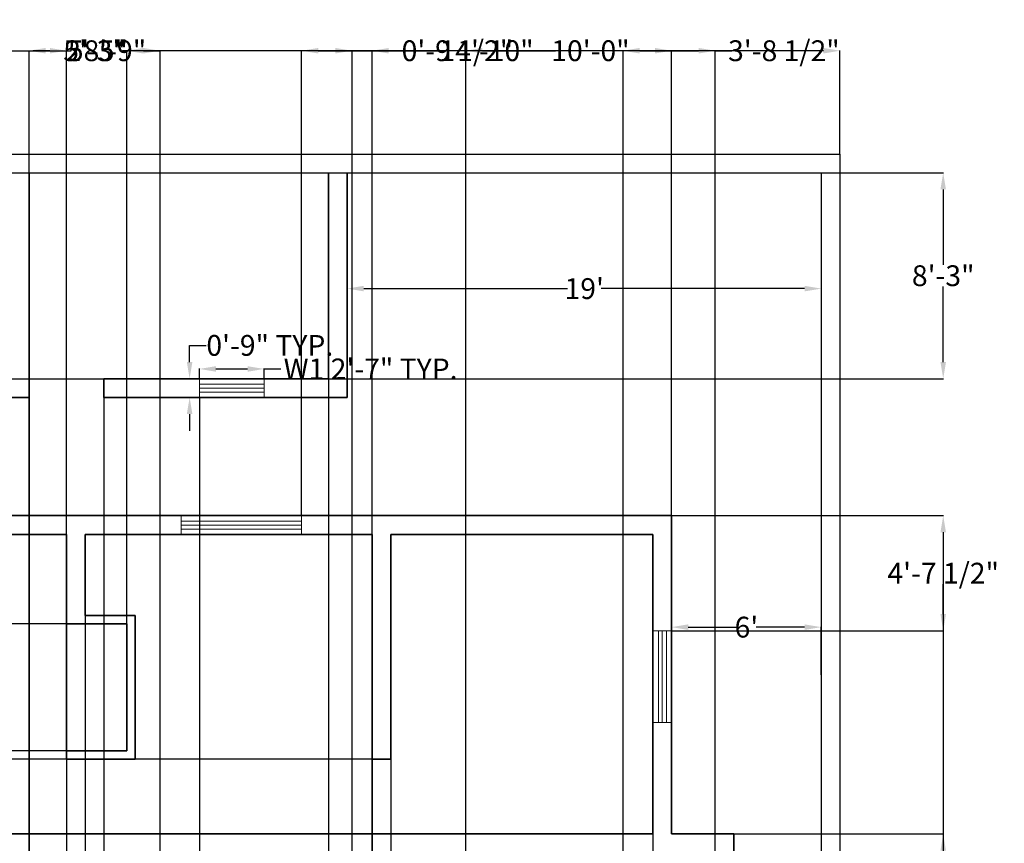
# Model space of a CAD drawing. Units: inches. Extents: x -63 to 800, y 3068 to 4133.
# Tile 5 of 5: x 327 to 800, y 3737 to 4133. Entities that reach past the tile are written whole.
import ezdxf

# ---------------------------------------------------------------- set-up
doc = ezdxf.new("R2010")
doc.units = ezdxf.units.IN
doc.header["$MEASUREMENT"] = 0
for name, color, linetype, lineweight in [('A-ANNO-DIMS', 2, 'Continuous', 13), ('A-GLAZ', 4, 'Continuous', 18), ('A-WALL', 7, 'Continuous', 35), ('A-WALL-SITE', 8, 'Continuous', 30)]:
    doc.layers.add(name, color=color, linetype=linetype, lineweight=lineweight)
doc.styles.get("Standard").update_dxf_attribs({"font": 'arial.ttf'})
doc.dimstyles.get("Standard").update_dxf_attribs({"dimtxt": 10, "dimasz": 8, "dimexe": 0.18, "dimexo": 0.0625, "dimgap": 0.09, "dimtad": 0, "dimtih": 1, "dimtoh": 1, "dimdec": 0, "dimzin": 0, "dimdsep": 46, "dimlunit": 3, "dimtxsty": 'Standard', "dimcen": 0.09, "dimadec": 0, "dimazin": 0, "dimtfac": 1, "dimtdec": 0, "dimtofl": 0, "dimtmove": 0, "dimatfit": 3, "dimfxl": 1, "dimtolj": 1, "dimtzin": 0, "dimarcsym": 0})

# ---------------------------------------------------------------- blocks, each defined once
blk = doc.blocks.new('*D1')
at = {"layer": 'A-ANNO-DIMS', "color": 0, "lineweight": -2, "transparency": 16777216}
for p, q in [((484.31, 4004.22), (484.31, 4003.78)), ((492.31, 4003.96), (590.2, 4003.96)), ((704.31, 4003.96), (606.41, 4003.96)), ((712.31, 4004.22), (712.31, 4003.78))]:
    blk.add_line(p, q, dxfattribs=at)
at = {"layer": 'A-ANNO-DIMS', "color": 0, "transparency": 16777216}
for points in [[(492.31, 4005.3), (492.31, 4002.63), (484.31, 4003.96)], [(704.31, 4005.3), (704.31, 4002.63), (712.31, 4003.96)]]:
    blk.add_solid(points, dxfattribs=at)
at = {"layer": 'Defpoints', "color": 0, "transparency": 16777216}
for p in [(484.31, 4004.28), (712.31, 4004.28), (712.31, 4003.96)]:
    blk.add_point(p, dxfattribs=at)
at = {"layer": 'A-ANNO-DIMS', "color": 0, "transparency": 16777216, "insert": (598.31, 4003.96), "char_height": 10, "attachment_point": 5}
blk.add_mtext("\\A1;19'", dxfattribs=at)
blk = doc.blocks.new('*D4')
at = {"layer": 'A-ANNO-DIMS', "color": 0, "lineweight": -2, "transparency": 16777216}
for p, q in [((640.31, 3818.37), (640.31, 3841.4)), ((648.31, 3841.22), (671.59, 3841.22)), ((704.31, 3841.22), (681.03, 3841.22)), ((712.31, 3818.37), (712.31, 3841.4))]:
    blk.add_line(p, q, dxfattribs=at)
at = {"layer": 'A-ANNO-DIMS', "color": 0, "transparency": 16777216}
for points in [[(648.31, 3842.55), (648.31, 3839.89), (640.31, 3841.22)], [(704.31, 3842.55), (704.31, 3839.89), (712.31, 3841.22)]]:
    blk.add_solid(points, dxfattribs=at)
at = {"layer": 'Defpoints', "color": 0, "transparency": 16777216}
for p in [(712.31, 3841.22), (640.31, 3818.31), (712.31, 3818.31)]:
    blk.add_point(p, dxfattribs=at)
at = {"layer": 'A-ANNO-DIMS', "color": 0, "transparency": 16777216, "insert": (676.31, 3841.22), "char_height": 10, "attachment_point": 5}
blk.add_mtext("\\A1;6'", dxfattribs=at)
blk = doc.blocks.new('WIN-31')
blk.add_lwpolyline([(0, 9), (31.17, 9), (31.17, 0), (0, 0)], close=True)
blk.add_lwpolyline([(0, 4.5), (31.17, 4.5), (31.17, 6.29), (0, 6.29), (0, 2.51), (31.17, 2.51)])
blk = doc.blocks.new('WIN-44')
blk.add_lwpolyline([(0, 0), (0, 44.17), (9, 44.17), (9, 0)], close=True)
for points in [[(2.71, 44.17), (2.71, 0), (6.5, 0), (6.5, 44.17)], [(4.5, 0), (4.5, 44.17)]]:
    blk.add_lwpolyline(points)
blk = doc.blocks.new('WIN-58')
blk.add_lwpolyline([(0, 9), (57.99, 9), (57.99, 0), (0, 0)], close=True)
for points in [[(0, 4.5), (57.99, 4.5), (57.99, 6.29), (0, 6.29)], [(0, 2.51), (57.99, 2.51)]]:
    blk.add_lwpolyline(points)
blk = doc.blocks.new('*D13')
at = {"layer": 'A-ANNO-DIMS', "color": 0, "lineweight": -2, "transparency": 16777216}
for p, q in [((413.21, 3960.72), (413.21, 3965.52)), ((421.21, 3965.34), (436.38, 3965.34)), ((444.38, 3960.72), (444.38, 3965.52)), ((444.38, 3965.34), (452.38, 3965.34))]:
    blk.add_line(p, q, dxfattribs=at)
at = {"layer": 'A-ANNO-DIMS', "color": 0, "transparency": 16777216}
for points in [[(421.21, 3966.67), (421.21, 3964), (413.21, 3965.34)], [(436.38, 3966.67), (436.38, 3964), (444.38, 3965.34)]]:
    blk.add_solid(points, dxfattribs=at)
at = {"layer": 'Defpoints', "color": 0, "transparency": 16777216}
for p in [(444.38, 3965.34), (413.21, 3960.66), (444.38, 3960.66)]:
    blk.add_point(p, dxfattribs=at)
at = {"layer": 'A-ANNO-DIMS', "color": 0, "transparency": 16777216, "insert": (495.58, 3965.34), "char_height": 10, "attachment_point": 5}
blk.add_mtext('\\A1;W1 2\'-7" TYP.', dxfattribs=at)
blk = doc.blocks.new('*D14')
at = {"layer": 'A-ANNO-DIMS', "color": 0, "lineweight": -2, "transparency": 16777216}
for p, q in [((408.54, 3968.66), (408.54, 3976.66)), ((408.54, 3976.66), (416.54, 3976.66)), ((413.15, 3960.66), (408.36, 3960.66)), ((413.15, 3951.66), (408.36, 3951.66)), ((408.54, 3943.66), (408.54, 3935.66))]:
    blk.add_line(p, q, dxfattribs=at)
at = {"layer": 'A-ANNO-DIMS', "color": 0, "transparency": 16777216}
for points in [[(407.2, 3968.66), (409.87, 3968.66), (408.54, 3960.66)], [(407.2, 3943.66), (409.87, 3943.66), (408.54, 3951.66)]]:
    blk.add_solid(points, dxfattribs=at)
at = {"layer": 'Defpoints', "color": 0, "transparency": 16777216}
for p in [(408.54, 3960.66), (413.21, 3960.66), (413.21, 3951.66)]:
    blk.add_point(p, dxfattribs=at)
at = {"layer": 'A-ANNO-DIMS', "color": 0, "transparency": 16777216, "insert": (447.1, 3976.66), "char_height": 10, "attachment_point": 5}
blk.add_mtext('\\A1;0\'-9" TYP.', dxfattribs=at)
blk = doc.blocks.new('*D19')
at = {"layer": 'A-ANNO-DIMS', "color": 0, "lineweight": -2, "transparency": 16777216}
for p, q in [((16.31, 4068.72), (16.31, 4118.49)), ((24.31, 4118.31), (351.54, 4118.31)), ((713.31, 4118.31), (386.08, 4118.31)), ((721.31, 4068.72), (721.31, 4118.49))]:
    blk.add_line(p, q, dxfattribs=at)
at = {"layer": 'A-ANNO-DIMS', "color": 0, "transparency": 16777216}
for points in [[(24.31, 4119.64), (24.31, 4116.98), (16.31, 4118.31)], [(713.31, 4119.64), (713.31, 4116.98), (721.31, 4118.31)]]:
    blk.add_solid(points, dxfattribs=at)
at = {"layer": 'Defpoints', "color": 0, "transparency": 16777216}
for p in [(721.31, 4118.31), (16.31, 4068.66), (721.31, 4068.66)]:
    blk.add_point(p, dxfattribs=at)
at = {"layer": 'A-ANNO-DIMS', "color": 0, "transparency": 16777216, "insert": (368.81, 4118.31), "char_height": 10, "attachment_point": 5}
blk.add_mtext('\\A1;58\'-9"', dxfattribs=at)
blk = doc.blocks.new('*D25')
at = {"layer": 'A-ANNO-DIMS', "color": 0, "lineweight": -2, "transparency": 16777216}
for p, q in [((331.31, 4059.6), (331.31, 3082.48)), ((475.31, 4059.6), (475.31, 3082.48)), ((339.31, 3082.66), (386.51, 3082.66)), ((467.31, 3082.66), (420.1, 3082.66))]:
    blk.add_line(p, q, dxfattribs=at)
at = {"layer": 'A-ANNO-DIMS', "color": 0, "transparency": 16777216}
for points in [[(339.31, 3083.99), (339.31, 3081.33), (331.31, 3082.66)], [(467.31, 3083.99), (467.31, 3081.33), (475.31, 3082.66)]]:
    blk.add_solid(points, dxfattribs=at)
at = {"layer": 'Defpoints', "color": 0, "transparency": 16777216}
for p in [(331.31, 4059.66), (475.31, 4059.66), (475.31, 3082.66)]:
    blk.add_point(p, dxfattribs=at)
at = {"layer": 'A-ANNO-DIMS', "color": 0, "transparency": 16777216, "insert": (403.31, 3082.66), "char_height": 10, "attachment_point": 5}
blk.add_mtext('\\A1;12\'-0"', dxfattribs=at)
blk = doc.blocks.new('*D26')
at = {"layer": 'A-ANNO-DIMS', "color": 0, "lineweight": -2, "transparency": 16777216}
for p, q in [((25.37, 4059.66), (771.14, 4059.66)), ((770.96, 4051.66), (770.96, 4015.36)), ((770.96, 3968.66), (770.96, 4004.96)), ((25.37, 3960.66), (771.14, 3960.66))]:
    blk.add_line(p, q, dxfattribs=at)
at = {"layer": 'A-ANNO-DIMS', "color": 0, "transparency": 16777216}
for points in [[(769.63, 4051.66), (772.29, 4051.66), (770.96, 4059.66)], [(769.63, 3968.66), (772.29, 3968.66), (770.96, 3960.66)]]:
    blk.add_solid(points, dxfattribs=at)
at = {"layer": 'Defpoints', "color": 0, "transparency": 16777216}
for p in [(25.31, 4059.66), (770.96, 4059.66), (25.31, 3960.66)]:
    blk.add_point(p, dxfattribs=at)
at = {"layer": 'A-ANNO-DIMS', "color": 0, "transparency": 16777216, "insert": (770.96, 4010.16), "char_height": 10, "attachment_point": 5}
blk.add_mtext('\\A1;8\'-3"', dxfattribs=at)
blk = doc.blocks.new('*D28')
at = {"layer": 'A-ANNO-DIMS', "color": 0, "lineweight": -2, "transparency": 16777216}
for p, q in [((297.16, 3951.55), (297.16, 3082.48)), ((331.31, 3951.6), (331.31, 3082.48)), ((305.16, 3082.66), (323.31, 3082.66)), ((331.31, 3082.66), (339.31, 3082.66))]:
    blk.add_line(p, q, dxfattribs=at)
at = {"layer": 'A-ANNO-DIMS', "color": 0, "transparency": 16777216}
for points in [[(305.16, 3083.99), (305.16, 3081.33), (297.16, 3082.66)], [(323.31, 3083.99), (323.31, 3081.33), (331.31, 3082.66)]]:
    blk.add_solid(points, dxfattribs=at)
at = {"layer": 'Defpoints', "color": 0, "transparency": 16777216}
for p in [(297.16, 3951.61), (331.31, 3951.66), (331.31, 3082.66)]:
    blk.add_point(p, dxfattribs=at)
at = {"layer": 'A-ANNO-DIMS', "color": 0, "transparency": 16777216, "insert": (356.66, 3082.66), "char_height": 10, "attachment_point": 5}
blk.add_mtext('\\A1;2\'-10"', dxfattribs=at)
blk = doc.blocks.new('*D29')
at = {"layer": 'A-ANNO-DIMS', "color": 0, "lineweight": -2, "transparency": 16777216}
for p, q in [((367.31, 3951.6), (367.31, 3082.48)), ((413.21, 3951.6), (413.21, 3082.48)), ((359.31, 3082.66), (351.31, 3082.66)), ((421.21, 3082.66), (429.21, 3082.66))]:
    blk.add_line(p, q, dxfattribs=at)
at = {"layer": 'A-ANNO-DIMS', "color": 0, "transparency": 16777216}
for points in [[(359.31, 3083.99), (359.31, 3081.33), (367.31, 3082.66)], [(421.21, 3083.99), (421.21, 3081.33), (413.21, 3082.66)]]:
    blk.add_solid(points, dxfattribs=at)
at = {"layer": 'Defpoints', "color": 0, "transparency": 16777216}
for p in [(367.31, 3951.66), (413.21, 3951.66), (413.21, 3082.66)]:
    blk.add_point(p, dxfattribs=at)
at = {"layer": 'A-ANNO-DIMS', "color": 0, "transparency": 16777216, "insert": (390.26, 3082.66), "char_height": 10, "attachment_point": 5}
blk.add_mtext('\\A1;3\'-10"', dxfattribs=at)
blk = doc.blocks.new('*D32')
at = {"layer": 'A-ANNO-DIMS', "color": 0, "lineweight": -2, "transparency": 16777216}
for p, q in [((331.31, 3951.6), (331.31, 3082.48)), ((367.31, 3951.6), (367.31, 3082.48)), ((323.31, 3082.66), (315.31, 3082.66)), ((375.31, 3082.66), (383.31, 3082.66))]:
    blk.add_line(p, q, dxfattribs=at)
at = {"layer": 'A-ANNO-DIMS', "color": 0, "transparency": 16777216}
for points in [[(323.31, 3083.99), (323.31, 3081.33), (331.31, 3082.66)], [(375.31, 3083.99), (375.31, 3081.33), (367.31, 3082.66)]]:
    blk.add_solid(points, dxfattribs=at)
at = {"layer": 'Defpoints', "color": 0, "transparency": 16777216}
for p in [(331.31, 3951.66), (367.31, 3951.66), (367.31, 3082.66)]:
    blk.add_point(p, dxfattribs=at)
at = {"layer": 'A-ANNO-DIMS', "color": 0, "transparency": 16777216, "insert": (349.31, 3082.66), "char_height": 10, "attachment_point": 5}
blk.add_mtext('\\A1;3\'-0"', dxfattribs=at)
blk = doc.blocks.new('*D35')
at = {"layer": 'A-ANNO-DIMS', "color": 0, "lineweight": -2, "transparency": 16777216}
for p, q in [((640.37, 3894.81), (771.14, 3894.81)), ((770.96, 3886.81), (770.96, 3608.32)), ((770.96, 3319.31), (770.96, 3597.8)), ((670.37, 3311.31), (771.14, 3311.31))]:
    blk.add_line(p, q, dxfattribs=at)
at = {"layer": 'A-ANNO-DIMS', "color": 0, "transparency": 16777216}
for points in [[(769.63, 3886.81), (772.29, 3886.81), (770.96, 3894.81)], [(769.63, 3319.31), (772.29, 3319.31), (770.96, 3311.31)]]:
    blk.add_solid(points, dxfattribs=at)
at = {"layer": 'Defpoints', "color": 0, "transparency": 16777216}
for p in [(640.31, 3894.81), (770.96, 3894.81), (670.31, 3311.31)]:
    blk.add_point(p, dxfattribs=at)
at = {"layer": 'A-ANNO-DIMS', "color": 0, "transparency": 16777216, "insert": (770.96, 3603.06), "char_height": 10, "attachment_point": 5}
blk.add_mtext('\\A1;48\'-7 1/2"', dxfattribs=at)
blk = doc.blocks.new('*D37')
at = {"layer": 'A-ANNO-DIMS', "color": 0, "lineweight": -2, "transparency": 16777216}
for p, q in [((181.31, 3885.75), (181.31, 3082.48)), ((349.31, 3885.75), (349.31, 3082.48)), ((189.31, 3082.66), (248.51, 3082.66)), ((341.31, 3082.66), (282.1, 3082.66))]:
    blk.add_line(p, q, dxfattribs=at)
at = {"layer": 'A-ANNO-DIMS', "color": 0, "transparency": 16777216}
for points in [[(189.31, 3083.99), (189.31, 3081.33), (181.31, 3082.66)], [(341.31, 3083.99), (341.31, 3081.33), (349.31, 3082.66)]]:
    blk.add_solid(points, dxfattribs=at)
at = {"layer": 'Defpoints', "color": 0, "transparency": 16777216}
for p in [(181.31, 3885.81), (349.31, 3885.81), (349.31, 3082.66)]:
    blk.add_point(p, dxfattribs=at)
at = {"layer": 'A-ANNO-DIMS', "color": 0, "transparency": 16777216, "insert": (265.31, 3082.66), "char_height": 10, "attachment_point": 5}
blk.add_mtext('\\A1;14\'-0"', dxfattribs=at)
blk = doc.blocks.new('*D38')
at = {"layer": 'A-ANNO-DIMS', "color": 0, "lineweight": -2, "transparency": 16777216}
for p, q in [((358.31, 3885.75), (358.31, 3082.48)), ((496.31, 3885.75), (496.31, 3082.48)), ((366.31, 3082.66), (410.51, 3082.66)), ((488.31, 3082.66), (444.1, 3082.66))]:
    blk.add_line(p, q, dxfattribs=at)
at = {"layer": 'A-ANNO-DIMS', "color": 0, "transparency": 16777216}
for points in [[(366.31, 3083.99), (366.31, 3081.33), (358.31, 3082.66)], [(488.31, 3083.99), (488.31, 3081.33), (496.31, 3082.66)]]:
    blk.add_solid(points, dxfattribs=at)
at = {"layer": 'Defpoints', "color": 0, "transparency": 16777216}
for p in [(358.31, 3885.81), (496.31, 3885.81), (496.31, 3082.66)]:
    blk.add_point(p, dxfattribs=at)
at = {"layer": 'A-ANNO-DIMS', "color": 0, "transparency": 16777216, "insert": (427.31, 3082.66), "char_height": 10, "attachment_point": 5}
blk.add_mtext('\\A1;11\'-6"', dxfattribs=at)
blk = doc.blocks.new('*D39')
at = {"layer": 'A-ANNO-DIMS', "color": 0, "lineweight": -2, "transparency": 16777216}
for p, q in [((505.31, 3885.75), (505.31, 3082.48)), ((631.31, 3885.75), (631.31, 3082.48)), ((513.31, 3082.66), (551.51, 3082.66)), ((623.31, 3082.66), (585.1, 3082.66))]:
    blk.add_line(p, q, dxfattribs=at)
at = {"layer": 'A-ANNO-DIMS', "color": 0, "transparency": 16777216}
for points in [[(513.31, 3083.99), (513.31, 3081.33), (505.31, 3082.66)], [(623.31, 3083.99), (623.31, 3081.33), (631.31, 3082.66)]]:
    blk.add_solid(points, dxfattribs=at)
at = {"layer": 'Defpoints', "color": 0, "transparency": 16777216}
for p in [(505.31, 3885.81), (631.31, 3885.81), (631.31, 3082.66)]:
    blk.add_point(p, dxfattribs=at)
at = {"layer": 'A-ANNO-DIMS', "color": 0, "transparency": 16777216, "insert": (568.31, 3082.66), "char_height": 10, "attachment_point": 5}
blk.add_mtext('\\A1;10\'-6"', dxfattribs=at)
blk = doc.blocks.new('*D41')
at = {"layer": 'A-ANNO-DIMS', "color": 0, "lineweight": -2, "transparency": 16777216}
for p, q in [((462.42, 3894.87), (462.42, 4118.49)), ((470.42, 4118.31), (530.68, 4118.31)), ((632.31, 4118.31), (572.04, 4118.31)), ((640.31, 3894.87), (640.31, 4118.49))]:
    blk.add_line(p, q, dxfattribs=at)
at = {"layer": 'A-ANNO-DIMS', "color": 0, "transparency": 16777216}
for points in [[(470.42, 4119.64), (470.42, 4116.98), (462.42, 4118.31)], [(632.31, 4119.64), (632.31, 4116.98), (640.31, 4118.31)]]:
    blk.add_solid(points, dxfattribs=at)
at = {"layer": 'Defpoints', "color": 0, "transparency": 16777216}
for p in [(640.31, 4118.31), (462.42, 3894.81), (640.31, 3894.81)]:
    blk.add_point(p, dxfattribs=at)
at = {"layer": 'A-ANNO-DIMS', "color": 0, "transparency": 16777216, "insert": (551.36, 4118.31), "char_height": 10, "attachment_point": 5}
blk.add_mtext('\\A1;14\'-10"', dxfattribs=at)
blk = doc.blocks.new('*D43')
at = {"layer": 'A-ANNO-DIMS', "color": 0, "lineweight": -2, "transparency": 16777216}
for p, q in [((640.37, 3894.81), (771.14, 3894.81)), ((770.96, 3886.81), (770.96, 3872.42)), ((770.96, 3847.51), (770.96, 3861.9)), ((640.37, 3839.51), (771.14, 3839.51))]:
    blk.add_line(p, q, dxfattribs=at)
at = {"layer": 'A-ANNO-DIMS', "color": 0, "transparency": 16777216}
for points in [[(769.63, 3886.81), (772.29, 3886.81), (770.96, 3894.81)], [(769.63, 3847.51), (772.29, 3847.51), (770.96, 3839.51)]]:
    blk.add_solid(points, dxfattribs=at)
at = {"layer": 'Defpoints', "color": 0, "transparency": 16777216}
for p in [(640.31, 3894.81), (770.96, 3894.81), (640.31, 3839.51)]:
    blk.add_point(p, dxfattribs=at)
at = {"layer": 'A-ANNO-DIMS', "color": 0, "transparency": 16777216, "insert": (770.96, 3867.16), "char_height": 10, "attachment_point": 5}
blk.add_mtext('\\A1;4\'-7 1/2"', dxfattribs=at)
blk = doc.blocks.new('*D50')
at = {"layer": 'A-ANNO-DIMS', "color": 0, "lineweight": -2, "transparency": 16777216}
for p, q in [((670.37, 3741.81), (771.14, 3741.81)), ((770.96, 3733.81), (770.96, 3719.88)), ((770.96, 3695.44), (770.96, 3709.36)), ((670.37, 3687.44), (771.14, 3687.44))]:
    blk.add_line(p, q, dxfattribs=at)
at = {"layer": 'A-ANNO-DIMS', "color": 0, "transparency": 16777216}
for points in [[(769.63, 3733.81), (772.29, 3733.81), (770.96, 3741.81)], [(769.63, 3695.44), (772.29, 3695.44), (770.96, 3687.44)]]:
    blk.add_solid(points, dxfattribs=at)
at = {"layer": 'Defpoints', "color": 0, "transparency": 16777216}
for p in [(670.31, 3741.81), (770.96, 3741.81), (670.31, 3687.44)]:
    blk.add_point(p, dxfattribs=at)
at = {"layer": 'A-ANNO-DIMS', "color": 0, "transparency": 16777216, "insert": (770.96, 3714.62), "char_height": 10, "attachment_point": 5}
blk.add_mtext('\\A1;4\'-6 1/2"', dxfattribs=at)
blk = doc.blocks.new('*D53')
at = {"layer": 'A-ANNO-DIMS', "color": 0, "lineweight": -2, "transparency": 16777216}
for p, q in [((541.31, 3594.87), (541.31, 4118.49)), ((549.31, 4118.31), (584.51, 4118.31)), ((653.31, 4118.31), (618.1, 4118.31)), ((661.31, 3594.87), (661.31, 4118.49))]:
    blk.add_line(p, q, dxfattribs=at)
at = {"layer": 'A-ANNO-DIMS', "color": 0, "transparency": 16777216}
for points in [[(549.31, 4119.64), (549.31, 4116.98), (541.31, 4118.31)], [(653.31, 4119.64), (653.31, 4116.98), (661.31, 4118.31)]]:
    blk.add_solid(points, dxfattribs=at)
at = {"layer": 'Defpoints', "color": 0, "transparency": 16777216}
for p in [(661.31, 4118.31), (541.31, 3594.81), (661.31, 3594.81)]:
    blk.add_point(p, dxfattribs=at)
at = {"layer": 'A-ANNO-DIMS', "color": 0, "transparency": 16777216, "insert": (601.31, 4118.31), "char_height": 10, "attachment_point": 5}
blk.add_mtext('\\A1;10\'-0"', dxfattribs=at)
blk = doc.blocks.new('*D58')
at = {"layer": 'A-ANNO-DIMS', "color": 0, "lineweight": -2, "transparency": 16777216}
for p, q in [((616.98, 3320.37), (616.98, 4118.49)), ((624.98, 4118.31), (653.31, 4118.31)), ((661.31, 3320.37), (661.31, 4118.49)), ((661.31, 4118.31), (669.31, 4118.31))]:
    blk.add_line(p, q, dxfattribs=at)
at = {"layer": 'A-ANNO-DIMS', "color": 0, "transparency": 16777216}
for points in [[(624.98, 4119.64), (624.98, 4116.98), (616.98, 4118.31)], [(653.31, 4119.64), (653.31, 4116.98), (661.31, 4118.31)]]:
    blk.add_solid(points, dxfattribs=at)
at = {"layer": 'Defpoints', "color": 0, "transparency": 16777216}
for p in [(661.31, 4118.31), (616.98, 3320.31), (661.31, 3320.31)]:
    blk.add_point(p, dxfattribs=at)
at = {"layer": 'A-ANNO-DIMS', "color": 0, "transparency": 16777216, "insert": (694.34, 4118.31), "char_height": 10, "attachment_point": 5}
blk.add_mtext('\\A1;3\'-8 1/2"', dxfattribs=at)
blk = doc.blocks.new('*D62')
at = {"layer": 'A-ANNO-DIMS', "color": 0, "lineweight": -2, "transparency": 16777216}
for p, q in [((478.66, 4118.31), (470.66, 4118.31)), ((486.66, 3473.37), (486.66, 4118.49)), ((496.31, 3473.37), (496.31, 4118.49)), ((504.31, 4118.31), (512.31, 4118.31))]:
    blk.add_line(p, q, dxfattribs=at)
at = {"layer": 'A-ANNO-DIMS', "color": 0, "transparency": 16777216}
for points in [[(478.66, 4119.64), (478.66, 4116.98), (486.66, 4118.31)], [(504.31, 4119.64), (504.31, 4116.98), (496.31, 4118.31)]]:
    blk.add_solid(points, dxfattribs=at)
at = {"layer": 'Defpoints', "color": 0, "transparency": 16777216}
for p in [(496.31, 4118.31), (486.66, 3473.31), (496.31, 3473.31)]:
    blk.add_point(p, dxfattribs=at)
at = {"layer": 'A-ANNO-DIMS', "color": 0, "transparency": 16777216, "insert": (537.34, 4118.31), "char_height": 10, "attachment_point": 5}
blk.add_mtext('\\A1;0\'-9 1/2"', dxfattribs=at)
blk = doc.blocks.new('*D65')
at = {"layer": 'A-ANNO-DIMS', "color": 0, "lineweight": -2, "transparency": 16777216}
for p, q in [((341.31, 4118.31), (333.31, 4118.31)), ((349.31, 3781.87), (349.31, 4118.49)), ((378.31, 3781.87), (378.31, 4118.49)), ((386.31, 4118.31), (394.31, 4118.31))]:
    blk.add_line(p, q, dxfattribs=at)
at = {"layer": 'A-ANNO-DIMS', "color": 0, "transparency": 16777216}
for points in [[(341.31, 4119.64), (341.31, 4116.98), (349.31, 4118.31)], [(386.31, 4119.64), (386.31, 4116.98), (378.31, 4118.31)]]:
    blk.add_solid(points, dxfattribs=at)
at = {"layer": 'Defpoints', "color": 0, "transparency": 16777216}
for p in [(378.31, 4118.31), (349.31, 3781.81), (378.31, 3781.81)]:
    blk.add_point(p, dxfattribs=at)
at = {"layer": 'A-ANNO-DIMS', "color": 0, "transparency": 16777216, "insert": (363.81, 4118.31), "char_height": 10, "attachment_point": 5}
blk.add_mtext('\\A1;2\'-5"', dxfattribs=at)
blk = doc.blocks.new('*D66')
at = {"layer": 'A-ANNO-DIMS', "color": 0, "lineweight": -2, "transparency": 16777216}
for p, q in [((378.25, 3842.81), (-33.52, 3842.81)), ((-33.34, 3834.81), (-33.34, 3817.51)), ((-33.34, 3789.81), (-33.34, 3807.11)), ((378.25, 3781.81), (-33.52, 3781.81))]:
    blk.add_line(p, q, dxfattribs=at)
at = {"layer": 'A-ANNO-DIMS', "color": 0, "transparency": 16777216}
for points in [[(-34.67, 3834.81), (-32.01, 3834.81), (-33.34, 3842.81)], [(-34.67, 3789.81), (-32.01, 3789.81), (-33.34, 3781.81)]]:
    blk.add_solid(points, dxfattribs=at)
at = {"layer": 'Defpoints', "color": 0, "transparency": 16777216}
for p in [(-33.34, 3842.81), (378.31, 3842.81), (378.31, 3781.81)]:
    blk.add_point(p, dxfattribs=at)
at = {"layer": 'A-ANNO-DIMS', "color": 0, "transparency": 16777216, "insert": (-33.34, 3812.31), "char_height": 10, "attachment_point": 5}
blk.add_mtext('\\A1;5\'-1"', dxfattribs=at)
blk = doc.blocks.new('*D67')
at = {"layer": 'A-ANNO-DIMS', "color": 0, "lineweight": -2, "transparency": 16777216}
for p, q in [((505.25, 3777.81), (-33.52, 3777.81)), ((-33.34, 3769.81), (-33.34, 3765.01)), ((-33.34, 3749.81), (-33.34, 3754.61)), ((631.25, 3741.81), (-33.52, 3741.81))]:
    blk.add_line(p, q, dxfattribs=at)
at = {"layer": 'A-ANNO-DIMS', "color": 0, "transparency": 16777216}
for points in [[(-34.67, 3769.81), (-32.01, 3769.81), (-33.34, 3777.81)], [(-34.67, 3749.81), (-32.01, 3749.81), (-33.34, 3741.81)]]:
    blk.add_solid(points, dxfattribs=at)
at = {"layer": 'Defpoints', "color": 0, "transparency": 16777216}
for p in [(505.31, 3777.81), (-33.34, 3741.81), (631.31, 3741.81)]:
    blk.add_point(p, dxfattribs=at)
at = {"layer": 'A-ANNO-DIMS', "color": 0, "transparency": 16777216, "insert": (-33.34, 3759.81), "char_height": 10, "attachment_point": 5}
blk.add_mtext('\\A1;3\'-0"', dxfattribs=at)
blk = doc.blocks.new('*D70')
at = {"layer": 'A-ANNO-DIMS', "color": 0, "lineweight": -2, "transparency": 16777216}
for p, q in [((331.31, 3263.37), (331.31, 4118.49)), ((339.31, 4118.31), (349.43, 4118.31)), ((386.31, 4118.31), (376.19, 4118.31)), ((394.31, 3263.37), (394.31, 4118.49))]:
    blk.add_line(p, q, dxfattribs=at)
at = {"layer": 'A-ANNO-DIMS', "color": 0, "transparency": 16777216}
for points in [[(339.31, 4119.64), (339.31, 4116.98), (331.31, 4118.31)], [(386.31, 4119.64), (386.31, 4116.98), (394.31, 4118.31)]]:
    blk.add_solid(points, dxfattribs=at)
at = {"layer": 'Defpoints', "color": 0, "transparency": 16777216}
for p in [(394.31, 4118.31), (331.31, 3263.31), (394.31, 3263.31)]:
    blk.add_point(p, dxfattribs=at)
at = {"layer": 'A-ANNO-DIMS', "color": 0, "transparency": 16777216, "insert": (362.81, 4118.31), "char_height": 10, "attachment_point": 5}
blk.add_mtext('\\A1;5\'-3"', dxfattribs=at)

msp = doc.modelspace()

# ---------------------------------------------------------------- linework, layer by layer
at = {"layer": 'A-WALL'}
for p, q in [((331.31, 4059.66), (331.31, 3951.66)), ((475.31, 4059.66), (475.31, 3960.66)), ((484.31, 4059.66), (484.31, 3951.66)), ((367.31, 3960.66), (475.31, 3960.66)), ((214.31, 3951.66), (331.31, 3951.66)), ((367.31, 3951.66), (484.31, 3951.66)), ((172.31, 3894.81), (640.31, 3894.81)), ((640.31, 3894.81), (640.31, 3741.81)), ((181.31, 3885.81), (349.31, 3885.81)), ((349.31, 3885.81), (349.31, 3842.81)), ((358.31, 3885.81), (358.31, 3846.81)), ((358.31, 3885.81), (382.31, 3885.81)), ((358.31, 3885.81), (496.31, 3885.81)), ((496.31, 3885.81), (496.31, 3777.81)), ((505.31, 3885.81), (505.31, 3777.81)), ((505.31, 3885.81), (631.31, 3885.81)), ((631.31, 3885.81), (631.31, 3741.81)), ((358.31, 3846.81), (382.31, 3846.81)), ((382.31, 3846.81), (382.31, 3777.81)), ((349.31, 3842.81), (378.31, 3842.81)), ((378.31, 3842.81), (378.31, 3781.81)), ((349.31, 3781.81), (378.31, 3781.81)), ((349.31, 3781.81), (349.31, 3777.81)), ((349.31, 3777.81), (382.31, 3777.81)), ((181.31, 3741.81), (496.31, 3741.81)), ((358.31, 3741.81), (378.31, 3741.81)), ((505.31, 3741.81), (631.31, 3741.81)), ((640.31, 3741.81), (670.31, 3741.81)), ((670.31, 3741.81), (670.31, 3263.31))]:
    msp.add_line(p, q, dxfattribs=at)
for points in [[(331.31, 3951.66), (331.31, 3960.66)], [(367.31, 3960.66), (367.31, 3951.66)], [(496.31, 3777.81), (505.31, 3777.81)], [(505.31, 3741.81), (505.31, 3741.81), (494.31, 3741.81)]]:
    msp.add_lwpolyline(points, dxfattribs=at)
at = {"layer": 'A-WALL-SITE'}
for p, q in [((16.31, 4068.66), (721.31, 4068.66)), ((721.31, 4068.66), (721.31, 3132.31)), ((331.31, 4059.66), (475.31, 4059.66)), ((484.31, 4059.66), (712.31, 4059.66)), ((712.31, 4059.66), (712.31, 3132.31))]:
    msp.add_line(p, q, dxfattribs=at)

# ---------------------------------------------------------------- block references
at = {"layer": 'A-GLAZ'}
for name, p in [('WIN-31', (413.21, 3951.66)), ('WIN-58', (404.42, 3885.81)), ('WIN-44', (631.31, 3795.34))]:
    msp.add_blockref(name, p, dxfattribs=at)

# ---------------------------------------------------------------- dimensions: what is measured, and where the dimension line sits
at = {"layer": 'A-ANNO-DIMS'}
for base, p1, p2, override, picture, middle in [((496.3095, 4118.3113), (486.6577, 3473.3102), (496.3095, 3473.3102), {"dimdec": 1, "dimlfac": 1, "dimrnd": 0, "dimzin": 1, "dimdsep": 46, "dimlunit": 4, "dimfrac": 2}, '*D62', (537.3415, 4118.3113)), ((661.31, 4118.31), (616.98, 3320.31), (661.31, 3320.31), {"dimdec": 1, "dimlfac": 1, "dimrnd": 0, "dimzin": 1, "dimdsep": 46, "dimlunit": 4, "dimfrac": 2}, '*D58', (694.34, 4118.31)), ((721.31, 4118.31), (16.31, 4068.66), (721.31, 4068.66), {"dimdec": 1, "dimlfac": 1, "dimrnd": 0, "dimzin": 1, "dimdsep": 46, "dimlunit": 4, "dimfrac": 2}, '*D19', (368.81, 4118.31)), ((394.31, 4118.31), (331.31, 3263.31), (394.31, 3263.31), {"dimdec": 1, "dimlfac": 1, "dimrnd": 0, "dimzin": 1, "dimdsep": 46, "dimlunit": 4, "dimfrac": 2}, '*D70', (362.81, 4118.31)), ((378.31, 4118.31), (349.31, 3781.81), (378.31, 3781.81), {"dimdec": 1, "dimlfac": 1, "dimrnd": 0, "dimzin": 1, "dimdsep": 46, "dimlunit": 4, "dimfrac": 2}, '*D65', (363.81, 4118.31)), ((640.31, 4118.31), (462.42, 3894.81), (640.31, 3894.81), {"dimdec": 1, "dimlfac": 1, "dimrnd": 0, "dimzin": 1, "dimdsep": 46, "dimlunit": 4, "dimfrac": 2}, '*D41', (551.36, 4118.31)), ((661.31, 4118.31), (541.31, 3594.81), (661.31, 3594.81), {"dimdec": 1, "dimlfac": 1, "dimrnd": 0, "dimzin": 1, "dimdsep": 46, "dimlunit": 4, "dimfrac": 2}, '*D53', (601.31, 4118.31)), ((475.31, 3082.66), (331.31, 4059.66), (475.31, 4059.66), {"dimdec": 1, "dimlfac": 1, "dimrnd": 0, "dimzin": 1, "dimdsep": 46, "dimlunit": 4, "dimfrac": 2}, '*D25', (403.31, 3082.66)), ((712.31, 4003.96), (484.31, 4004.28), (712.31, 4004.28), {"dimclrd": 0, "dimclre": 0, "dimclrt": 0}, '*D1', (598.31, 4003.96)), ((331.3095, 3082.6602), (297.1617, 3951.6131), (331.3095, 3951.6613), {"dimdec": 1, "dimlfac": 1, "dimrnd": 0, "dimzin": 1, "dimdsep": 46, "dimlunit": 4, "dimfrac": 2}, '*D28', (356.6607, 3082.6602)), ((367.31, 3082.66), (331.31, 3951.66), (367.31, 3951.66), {"dimdec": 1, "dimlfac": 1, "dimrnd": 0, "dimzin": 1, "dimdsep": 46, "dimlunit": 4, "dimfrac": 2}, '*D32', (349.31, 3082.66)), ((413.21, 3082.66), (367.31, 3951.66), (413.21, 3951.66), {"dimdec": 1, "dimlfac": 1, "dimrnd": 0, "dimzin": 1, "dimdsep": 46, "dimlunit": 4, "dimfrac": 2}, '*D29', (390.26, 3082.66)), ((349.31, 3082.66), (181.31, 3885.81), (349.31, 3885.81), {"dimdec": 1, "dimlfac": 1, "dimrnd": 0, "dimzin": 1, "dimdsep": 46, "dimlunit": 4, "dimfrac": 2}, '*D37', (265.31, 3082.66)), ((496.31, 3082.66), (358.31, 3885.81), (496.31, 3885.81), {"dimdec": 1, "dimlfac": 1, "dimrnd": 0, "dimzin": 1, "dimdsep": 46, "dimlunit": 4, "dimfrac": 2}, '*D38', (427.31, 3082.66)), ((631.31, 3082.66), (505.31, 3885.81), (631.31, 3885.81), {"dimdec": 1, "dimlfac": 1, "dimrnd": 0, "dimzin": 1, "dimdsep": 46, "dimlunit": 4, "dimfrac": 2}, '*D39', (568.31, 3082.66)), ((712.31, 3841.22), (640.31, 3818.31), (712.31, 3818.31), {"dimclrd": 0, "dimclre": 0, "dimclrt": 0}, '*D4', (676.31, 3841.22))]:
    dim = msp.add_linear_dim(base=base, p1=p1, p2=p2, dimstyle='Standard', override=override, dxfattribs=at)
    dim.commit()
    dim.dimension.update_dxf_attribs({"geometry": picture, "text_midpoint": middle})
for base, p1, p2, picture, middle in [((770.96, 4059.66), (25.31, 3960.66), (25.31, 4059.66), '*D26', (770.96, 4010.16)), ((770.96, 3894.81), (670.31, 3311.31), (640.31, 3894.81), '*D35', (770.96, 3603.06)), ((770.96, 3894.81), (640.31, 3839.51), (640.31, 3894.81), '*D43', (770.96, 3867.16)), ((-33.34, 3842.81), (378.31, 3781.81), (378.31, 3842.81), '*D66', (-33.34, 3812.31)), ((-33.34, 3741.81), (505.31, 3777.81), (631.31, 3741.81), '*D67', (-33.34, 3759.81)), ((770.96, 3741.81), (670.31, 3687.44), (670.31, 3741.81), '*D50', (770.96, 3714.62))]:
    dim = msp.add_linear_dim(base=base, p1=p1, p2=p2, angle=90, dimstyle='Standard', override={"dimdec": 1, "dimlfac": 1, "dimrnd": 0, "dimzin": 1, "dimdsep": 46, "dimlunit": 4, "dimfrac": 2}, dxfattribs=at)
    dim.commit()
    dim.dimension.update_dxf_attribs({"geometry": picture, "text_midpoint": middle})
dim = msp.add_linear_dim(base=(408.54, 3960.66), p1=(413.21, 3951.66), p2=(413.21, 3960.66), angle=90, text='<> TYP.', dimstyle='Standard', override={"dimdec": 1, "dimlfac": 1, "dimrnd": 0, "dimzin": 1, "dimdsep": 46, "dimlunit": 4, "dimfrac": 2}, dxfattribs=at)
dim.commit()
dim.dimension.update_dxf_attribs({"geometry": '*D14', "text_midpoint": (447.1, 3976.66)})
dim = msp.add_linear_dim(base=(444.38, 3965.34), p1=(413.21, 3960.66), p2=(444.38, 3960.66), text='W1 <> TYP.', dimstyle='Standard', override={"dimdec": 1, "dimlfac": 1, "dimrnd": 0, "dimzin": 1, "dimdsep": 46, "dimlunit": 4, "dimfrac": 2}, dxfattribs=at)
dim.commit()
dim.dimension.update_dxf_attribs({"geometry": '*D13', "text_midpoint": (495.58, 3965.34)})

doc.saveas('drawing.dxf')
